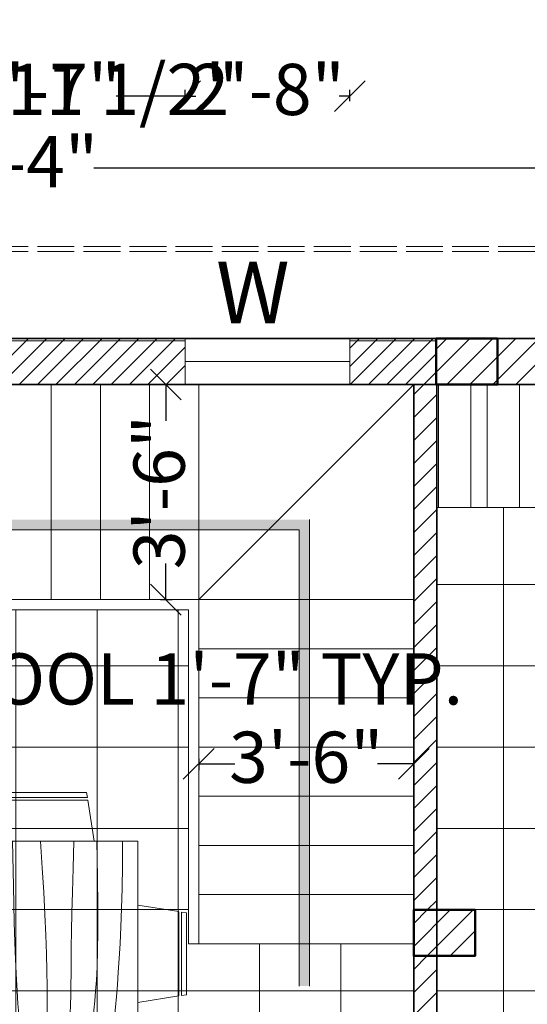
# Model space of a CAD drawing. Units: inches. Extents: x 2036 to 2670, y 319 to 920.
# Tile 11 of 15: x 2350 to 2449, y 728 to 920. Entities that reach past the tile are written whole.
import ezdxf

# ---------------------------------------------------------------- set-up
doc = ezdxf.new("R2010")
doc.units = ezdxf.units.IN
doc.linetypes.add('ACAD_ISO02W100', pattern=[15, 12, -3])
for name, color, linetype, lineweight in [('A-ANNO-DIMS', 2, 'Continuous', 18), ('A-ANNO-SYMB', 7, 'Continuous', 18), ('A-ANNO-SYMB-PATT', 7, 'Continuous', 13), ('A-ANNO-TEXT', 7, 'Continuous', 18), ('A-CASE', 7, 'Continuous', 18), ('A-CASE-PATT', 9, 'Continuous', 13), ('A-COLS', 7, 'Continuous', 50), ('A-FLOR-OVHD', 1, 'ACAD_ISO02W100', 13), ('A-FLOR-PATT', 8, 'Continuous', 9), ('A-FLOR-STRS', 7, 'Continuous', 18), ('A-FURN', 8, 'Continuous', 18), ('A-GLAZ', 4, 'Continuous', 18), ('A-WALL', 7, 'Continuous', 35)]:
    doc.layers.add(name, color=color, linetype=linetype, lineweight=lineweight)
doc.layers.add('A-COLS-PATT', color=240, linetype='Continuous', lineweight=13, true_color=0xed1f24)
doc.layers.add('A-WALL-PATT', color=52, linetype='Continuous', lineweight=13, true_color=0xc8c92d)
doc.styles.get("Standard").update_dxf_attribs({"font": 'arial.ttf'})
doc.dimstyles.new('ISO-25', dxfattribs={"dimtxt": 10, "dimasz": 6, "dimexe": 1.25, "dimexo": 0.625, "dimtad": 0, "dimdec": 1, "dimlunit": 3, "dimtxsty": 'Standard', "dimblk": 'OBLIQUE', "dimcen": 2.5, "dimclrd": 94, "dimclre": 94, "dimclrt": 1, "dimadec": 0, "dimazin": 0, "dimtfac": 1, "dimtdec": 1, "dimtmove": 0, "dimatfit": 3, "dimfxl": 1, "dimfxlon": 1, "dimarcsym": 0})

# ---------------------------------------------------------------- blocks, each defined once
blk = doc.blocks.new('Dining Set - 36 x 72 in.')
for p, q in [((-22, 27.5), (-22.1562, 26.50042)), ((-22, 27.5), (-6, 27.5)), ((-5.8437, 26.49966), (-6, 27.5)), ((6, 27.5), (5.8438, 26.50042)), ((6, 27.5), (22, 27.5)), ((22.1563, 26.49966), (22, 27.5)), ((-22.2343, 26.00059), (-23.4847, 17.99762)), ((-22.2304, 26), (-5.7608, 26)), ((-5.8416, 26.5), (-22.1534, 26.5)), ((-4.5152, 17.99762), (-5.7655, 25.99926)), ((5.7657, 26.00059), (4.5153, 17.99762)), ((5.7696, 26), (22.2392, 26)), ((22.1584, 26.5), (5.8466, 26.5)), ((23.4848, 17.99762), (22.2345, 25.99926)), ((36, 18), (-36, 18)), ((-36, 18), (-36, -18)), ((36, -18), (36, 18)), ((-45.5, 8), (-44.5004, 8.15617)), ((-45.5, 8), (-45.5, -8)), ((-44.5, -8.15843), (-44.5, 8.15338)), ((-44.0006, 8.23428), (-35.9976, 9.48474)), ((-44, 8.23041), (-44, -8.23915)), ((44.0006, 8.23428), (35.9976, 9.48474)), ((44, 8.23041), (44, -8.23915)), ((44.5, -8.15843), (44.5, 8.15338)), ((45.5, 8), (44.5005, 8.15617)), ((45.5, 8), (45.5, -8)), ((-44.4997, -8.15631), (-45.5, -8)), ((-35.9976, -9.48476), (-43.9993, -8.2345)), ((35.9976, -9.48476), (43.9993, -8.2345)), ((44.4997, -8.15631), (45.5, -8)), ((-36, -18), (36, -18)), ((-22.2343, -26.0006), (-23.4847, -17.99762)), ((-4.5152, -17.99762), (-5.7655, -25.99928)), ((5.7657, -26.0006), (4.5153, -17.99762)), ((23.4848, -17.99762), (22.2345, -25.99928)), ((-22.2304, -26), (-5.7608, -26)), ((-22, -27.5), (-22.1562, -26.50044)), ((-5.8416, -26.5), (-22.1534, -26.5)), ((-5.8437, -26.49967), (-6, -27.5)), ((5.7696, -26), (22.2392, -26)), ((6, -27.5), (5.8438, -26.50044)), ((22.1584, -26.5), (5.8466, -26.5)), ((22.1563, -26.49967), (22, -27.5)), ((-22, -27.5), (-6, -27.5)), ((6, -27.5), (22, -27.5))]:
    blk.add_line(p, q)
for points in [[(-36, 15), (-31.1772, 14.97754), (-26.8079, 14.91406), (-22.8538, 14.81543), (-19.276, 14.6875), (-16.0362, 14.53613), (-13.0957, 14.36718), (-10.4159, 14.18652), (-7.9583, 14), (-5.6904, 13.81315), (-3.6035, 13.63021), (-1.6954, 13.45508), (0.0365, 13.29166), (1.5945, 13.14388), (2.9811, 13.01562), (4.1988, 12.9108), (5.25, 12.83333), (6.1393, 12.78613), (6.8802, 12.76823), (7.4883, 12.77767), (7.9792, 12.8125), (8.3685, 12.87077), (8.6719, 12.95052), (8.9049, 13.0498), (9.0833, 13.16666), (9.2205, 13.29899), (9.3216, 13.44401), (9.3895, 13.59879), (9.4271, 13.76041), (9.4373, 13.92594), (9.4232, 14.09245), (9.3875, 14.257), (9.3333, 14.41666), (9.2638, 14.56917), (9.1836, 14.71484), (9.0975, 14.85465), (9.0104, 14.98958), (8.9272, 15.1206), (8.8529, 15.2487), (8.7922, 15.37483), (8.75, 15.5), (8.7305, 15.62467), (8.7344, 15.74739), (8.7617, 15.86621), (8.8125, 15.97916), (8.8867, 16.08431), (8.9844, 16.17968), (9.1055, 16.26334), (9.25, 16.33333), (9.4189, 16.38802), (9.6172, 16.42708), (9.8506, 16.45052), (10.125, 16.45833), (10.4463, 16.45052), (10.8203, 16.42708), (11.2529, 16.38802), (11.75, 16.33333), (12.3184, 16.26318), (12.9694, 16.17838), (13.7151, 16.07991), (14.5677, 15.96875), (15.5395, 15.84586), (16.6426, 15.71224), (17.8893, 15.56884), (19.2917, 15.41666), (20.859, 15.25667), (22.5879, 15.08984), (24.4721, 14.91715), (26.5052, 14.73958), (28.6809, 14.5581), (30.9929, 14.3737), (33.4347, 14.18733), (36, 14)], [(-36, 10), (-28.9766, 10.14274), (-23.1725, 10.20442), (-18.4241, 10.19775), (-14.5677, 10.13541), (-11.4399, 10.03011), (-8.877, 9.89453), (-6.7154, 9.74137), (-4.7917, 9.58333), (-2.9698, 9.43082), (-1.2246, 9.28515), (0.4415, 9.14534), (2.026, 9.01041), (3.5266, 8.87939), (4.9408, 8.7513), (6.266, 8.62516), (7.5, 8.5), (8.6411, 8.37549), (9.6914, 8.2539), (10.6538, 8.13818), (11.5312, 8.03125), (12.3267, 7.93603), (13.043, 7.85547), (13.6831, 7.79248), (14.25, 7.75), (14.7471, 7.7303), (15.1797, 7.73307), (15.5537, 7.75732), (15.875, 7.80208), (16.1494, 7.86637), (16.3828, 7.94922), (16.5811, 8.04964), (16.75, 8.16666), (16.8944, 8.29915), (17.0143, 8.44531), (17.1089, 8.60319), (17.1771, 8.77083), (17.218, 8.94629), (17.2305, 9.1276), (17.2137, 9.31282), (17.1667, 9.5), (17.0895, 9.6875), (16.987, 9.875), (16.8649, 10.0625), (16.7292, 10.25), (16.5856, 10.4375), (16.4401, 10.625), (16.2985, 10.8125), (16.1667, 11), (16.05, 11.18733), (15.9518, 11.3737), (15.8752, 11.5581), (15.8229, 11.73958), (15.798, 11.91715), (15.8034, 12.08984), (15.842, 12.25667), (15.9167, 12.41666), (16.0295, 12.56836), (16.1784, 12.70833), (16.3605, 12.83268), (16.5729, 12.9375), (16.8127, 13.01888), (17.0768, 13.07291), (17.3625, 13.0957), (17.6667, 13.08333), (17.9894, 13.03312), (18.3418, 12.94726), (18.7382, 12.82918), (19.1927, 12.68229), (19.7195, 12.51001), (20.3327, 12.31575), (21.0465, 12.10294), (21.875, 11.875), (22.8357, 11.63354), (23.959, 11.37304), (25.2786, 11.08618), (26.8282, 10.76562), (28.6414, 10.40405), (30.752, 9.99414), (33.1936, 9.52856), (36, 9)], [(-36, 5.5), (-30.7157, 5.3348), (-26.069, 5.20963), (-21.9946, 5.11767), (-18.4271, 5.05208), (-15.3009, 5.00602), (-12.5508, 4.97265), (-10.1112, 4.94515), (-7.9167, 4.91666), (-5.909, 4.88167), (-4.0586, 4.83984), (-2.3429, 4.79215), (-0.7396, 4.73958), (0.7739, 4.6831), (2.22, 4.6237), (3.6213, 4.56233), (5, 4.5), (6.373, 4.43782), (7.7344, 4.3776), (9.0723, 4.32129), (10.375, 4.27083), (11.6309, 4.22819), (12.8281, 4.19531), (13.9551, 4.17415), (15, 4.16666), (15.954, 4.17448), (16.819, 4.19791), (17.6001, 4.23698), (18.3021, 4.29166), (18.9299, 4.36198), (19.4883, 4.44791), (19.9823, 4.54948), (20.4167, 4.66666), (20.7969, 4.79899), (21.1302, 4.94401), (21.4245, 5.09879), (21.6875, 5.26041), (21.9271, 5.42594), (22.1511, 5.59245), (22.3672, 5.757), (22.5834, 5.91666), (22.8065, 6.06868), (23.0404, 6.21093), (23.2879, 6.34147), (23.5521, 6.45833), (23.8358, 6.55957), (24.142, 6.64323), (24.4735, 6.70735), (24.8334, 6.75), (25.2235, 6.76969), (25.642, 6.76692), (26.0858, 6.74267), (26.5521, 6.69791), (27.0379, 6.63362), (27.5404, 6.55078), (28.0565, 6.45036), (28.5834, 6.33333), (29.1242, 6.19987), (29.7071, 6.04687), (30.3661, 5.87044), (31.1354, 5.66666), (32.0493, 5.43164), (33.142, 5.16146), (34.4475, 4.85221), (36, 4.5)], [(-36, -1), (-30.7915, -0.6591), (-26.0195, -0.38216), (-21.6519, -0.16284), (-17.6563, 0.00521), (-14.0005, 0.12833), (-10.6523, 0.21289), (-7.5796, 0.26522), (-4.75, 0.29166), (-2.134, 0.29793), (0.2878, 0.28711), (2.5317, 0.26163), (4.6146, 0.22396), (6.5529, 0.17651), (8.3633, 0.12174), (10.0623, 0.06209), (11.6667, 0), (13.1899, -0.06201), (14.6341, -0.1211), (15.9982, -0.17432), (17.2813, -0.21875), (18.4823, -0.25147), (19.6003, -0.26953), (20.6343, -0.27002), (21.5834, -0.25), (22.4481, -0.20768), (23.2357, -0.14584), (23.9549, -0.06836), (24.6146, 0.02083), (25.2235, 0.11784), (25.7904, 0.21875), (26.3241, 0.31966), (26.8334, 0.41666), (27.3265, 0.50618), (27.8099, 0.58593), (28.2894, 0.65397), (28.7709, 0.70833), (29.2601, 0.74707), (29.763, 0.76823), (30.2855, 0.76985), (30.8334, 0.75), (31.4088, 0.70784), (31.9994, 0.64713), (32.589, 0.57275), (33.1615, 0.48958), (33.7008, 0.4025), (34.1908, 0.3164), (34.6153, 0.23616), (34.9584, 0.16666), (35.2099, 0.11165), (35.3848, 0.07031), (35.504, 0.04069), (35.5886, 0.02083), (35.6594, 0.00879), (35.7377, 0.0026), (35.8442, 0.00032), (36, 0)], [(-36, -6.5), (-27.1843, -6.31267), (-20.084, -6.1263), (-14.469, -5.9419), (-10.1094, -5.76042), (-6.7752, -5.58285), (-4.2363, -5.41016), (-2.2629, -5.24333), (-0.625, -5.08334), (0.8708, -4.93099), (2.2715, -4.78646), (3.5872, -4.64974), (4.8281, -4.52084), (6.0046, -4.39974), (7.127, -4.28646), (8.2053, -4.18099), (9.25, -4.08334), (10.2705, -3.99382), (11.2734, -3.91407), (12.2647, -3.84603), (13.25, -3.79167), (14.2354, -3.75293), (15.2266, -3.73177), (16.2295, -3.73015), (17.25, -3.75), (18.2912, -3.79248), (19.3451, -3.85547), (20.4009, -3.93604), (21.4479, -4.03125), (22.4754, -4.13819), (23.4727, -4.25391), (24.4289, -4.37549), (25.3334, -4.5), (26.1785, -4.62492), (26.9694, -4.74935), (27.7145, -4.87281), (28.4219, -4.99479), (29.1, -5.11483), (29.7572, -5.23242), (30.4016, -5.34709), (31.0417, -5.45834), (31.6837, -5.56437), (32.3262, -5.65821), (32.9658, -5.73153), (33.599, -5.77604), (34.2224, -5.78345), (34.8327, -5.74545), (35.4264, -5.65373), (36, -5.5)], [(-36, -10), (-26.4022, -9.81299), (-18.4675, -9.62891), (-11.9839, -9.45069), (-6.7396, -9.28125), (-2.5226, -9.12354), (0.8789, -8.98047), (3.6769, -8.85498), (6.0833, -8.75), (8.2767, -8.66765), (10.3021, -8.60677), (12.1712, -8.56543), (13.8958, -8.54167), (15.4876, -8.53353), (16.9583, -8.53907), (18.3197, -8.55632), (19.5834, -8.58334), (20.7616, -8.61841), (21.8685, -8.66081), (22.9188, -8.71004), (23.9271, -8.76563), (24.9081, -8.82707), (25.8763, -8.89388), (26.8465, -8.96558), (27.8334, -9.04167), (28.8474, -9.12118), (29.8828, -9.20117), (30.93, -9.27824), (31.9792, -9.34896), (33.0205, -9.40991), (34.0443, -9.45768), (35.0407, -9.48885), (36, -9.5)], [(-36, -14.5), (-30.0881, -14.33513), (-25.0332, -14.21224), (-20.7312, -14.12647), (-17.0781, -14.07292), (-13.97, -14.04671), (-11.3027, -14.04297), (-8.9724, -14.05681), (-6.875, -14.08334), (-4.9224, -14.11833), (-3.0905, -14.16016), (-1.3709, -14.20785), (0.2448, -14.26042), (1.7647, -14.3169), (3.1973, -14.3763), (4.5507, -14.43767), (5.8333, -14.5), (7.0554, -14.5621), (8.235, -14.62175), (9.3922, -14.67652), (10.5469, -14.72396), (11.7192, -14.76164), (12.929, -14.78711), (14.1965, -14.79794), (15.5417, -14.79167), (16.9933, -14.76424), (18.6152, -14.70508), (20.4804, -14.60197), (22.6615, -14.44271), (25.2312, -14.21509), (28.2624, -13.9069), (31.8277, -13.50594), (36, -13)]]:
    blk.add_lwpolyline(points)
blk = doc.blocks.new('_Oblique')
at = {"color": 0, "linetype": 'ByBlock', "lineweight": -2}
blk.add_line((-0.5, -0.5), (0.5, 0.5), dxfattribs=at)
blk = doc.blocks.new('*D10')
at = {"layer": 'A-ANNO-DIMS', "color": 0, "lineweight": -2, "transparency": 16777216}
for p, q in [((2080.74, 889.93), (2080.74, 892.18)), ((2080.74, 890.93), (2328.73, 890.93)), ((2612.74, 890.93), (2364.74, 890.93)), ((2612.74, 889.93), (2612.74, 892.18))]:
    blk.add_line(p, q, dxfattribs=at)
at = {"layer": 'Defpoints', "color": 0, "transparency": 16777216}
for p in [(2612.74, 890.93), (2080.74, 875.68), (2612.74, 875.68)]:
    blk.add_point(p, dxfattribs=at)
at = {"layer": 'A-ANNO-DIMS', "color": 0, "lineweight": -2, "transparency": 16777216, "xscale": 6, "yscale": 6, "zscale": 6, "rotation": 180}
blk.add_blockref('_Oblique', (2080.74, 890.93), dxfattribs=at)
at = {"layer": 'A-ANNO-DIMS', "color": 0, "lineweight": -2, "transparency": 16777216, "xscale": 6, "yscale": 6, "zscale": 6}
blk.add_blockref('_Oblique', (2612.74, 890.93), dxfattribs=at)
at = {"layer": 'A-ANNO-DIMS', "color": 0, "transparency": 16777216, "insert": (2346.74, 890.93), "char_height": 10, "attachment_point": 5}
blk.add_mtext('44\'-4"', dxfattribs=at)
blk = doc.blocks.new('*D16')
at = {"layer": 'A-ANNO-DIMS', "color": 0, "lineweight": -2, "transparency": 16777216}
for p, q in [((2377.81, 848.68), (2380.06, 848.68)), ((2378.81, 848.68), (2378.81, 841.6)), ((2378.81, 806.68), (2378.81, 813.77)), ((2377.81, 806.68), (2380.06, 806.68))]:
    blk.add_line(p, q, dxfattribs=at)
at = {"layer": 'Defpoints', "color": 0, "transparency": 16777216}
for p in [(2375.64, 848.68), (2378.81, 848.68), (2375.64, 806.68)]:
    blk.add_point(p, dxfattribs=at)
at = {"layer": 'A-ANNO-DIMS', "color": 0, "lineweight": -2, "transparency": 16777216, "xscale": 6, "yscale": 6, "zscale": 6}
for p, rotation in [((2378.81, 848.68), 90), ((2378.81, 806.68), 270)]:
    blk.add_blockref('_Oblique', p, dxfattribs=dict(at, rotation=rotation))
at = {"layer": 'A-ANNO-DIMS', "color": 0, "transparency": 16777216, "insert": (2378.81, 827.68), "char_height": 10, "attachment_point": 5, "rotation": 90}
blk.add_mtext('3\'-6"', dxfattribs=at)
blk = doc.blocks.new('*D17')
at = {"layer": 'A-ANNO-DIMS', "color": 0, "lineweight": -2, "transparency": 16777216}
for p, q in [((2385.24, 775.6), (2385.24, 773.35)), ((2427.24, 775.6), (2427.24, 773.35)), ((2385.24, 774.6), (2392.32, 774.6)), ((2427.24, 774.6), (2420.15, 774.6))]:
    blk.add_line(p, q, dxfattribs=at)
at = {"layer": 'Defpoints', "color": 0, "transparency": 16777216}
for p in [(2385.24, 777.88), (2427.24, 777.88), (2427.24, 774.6)]:
    blk.add_point(p, dxfattribs=at)
at = {"layer": 'A-ANNO-DIMS', "color": 0, "lineweight": -2, "transparency": 16777216, "xscale": 6, "yscale": 6, "zscale": 6, "rotation": 180}
blk.add_blockref('_Oblique', (2385.24, 774.6), dxfattribs=at)
at = {"layer": 'A-ANNO-DIMS', "color": 0, "lineweight": -2, "transparency": 16777216, "xscale": 6, "yscale": 6, "zscale": 6}
blk.add_blockref('_Oblique', (2427.24, 774.6), dxfattribs=at)
at = {"layer": 'A-ANNO-DIMS', "color": 0, "transparency": 16777216, "insert": (2406.24, 774.6), "char_height": 10, "attachment_point": 5}
blk.add_mtext('3\'-6"', dxfattribs=at)
blk = doc.blocks.new('COL-9x12')
blk.add_lwpolyline([(9, 0), (0, 0), (0, 12), (9, 12)], close=True)
blk = doc.blocks.new('*D27')
at = {"layer": 'A-ANNO-DIMS', "color": 94, "lineweight": -2, "transparency": 16777216}
for p, q in [((2300.93, 790.9), (2300.93, 788.65)), ((2320.17, 790.9), (2320.17, 788.65)), ((2300.93, 789.9), (2320.17, 789.9)), ((2320.17, 789.9), (2326.17, 789.9))]:
    blk.add_line(p, q, dxfattribs=at)
at = {"layer": 'Defpoints', "color": 0, "transparency": 16777216}
for p in [(2300.93, 792.79), (2320.17, 792.79), (2320.17, 789.9)]:
    blk.add_point(p, dxfattribs=at)
at = {"layer": 'A-ANNO-DIMS', "color": 94, "lineweight": -2, "transparency": 16777216, "xscale": 6, "yscale": 6, "zscale": 6, "rotation": 180}
blk.add_blockref('_Oblique', (2300.93, 789.9), dxfattribs=at)
at = {"layer": 'A-ANNO-DIMS', "color": 94, "lineweight": -2, "transparency": 16777216, "xscale": 6, "yscale": 6, "zscale": 6}
blk.add_blockref('_Oblique', (2320.17, 789.9), dxfattribs=at)
at = {"layer": 'A-ANNO-DIMS', "color": 1, "transparency": 16777216, "insert": (2382.86, 789.9), "char_height": 10, "attachment_point": 5}
blk.add_mtext('STOOL 1\'-7" TYP.', dxfattribs=at)
blk = doc.blocks.new('*D51')
at = {"layer": 'A-ANNO-DIMS', "color": 94, "lineweight": -2, "transparency": 16777216}
for p, q in [((2304.05, 904.03), (2304.05, 906.28)), ((2327.38, 904.03), (2327.38, 906.28)), ((2304.05, 905.03), (2327.38, 905.03)), ((2327.38, 905.03), (2333.38, 905.03))]:
    blk.add_line(p, q, dxfattribs=at)
at = {"layer": 'Defpoints', "color": 0, "transparency": 16777216}
for p in [(2327.38, 905.03), (2304.05, 857.68), (2327.38, 857.68)]:
    blk.add_point(p, dxfattribs=at)
at = {"layer": 'A-ANNO-DIMS', "color": 94, "lineweight": -2, "transparency": 16777216, "xscale": 6, "yscale": 6, "zscale": 6, "rotation": 180}
blk.add_blockref('_Oblique', (2304.05, 905.03), dxfattribs=at)
at = {"layer": 'A-ANNO-DIMS', "color": 94, "lineweight": -2, "transparency": 16777216, "xscale": 6, "yscale": 6, "zscale": 6}
blk.add_blockref('_Oblique', (2327.38, 905.03), dxfattribs=at)
at = {"layer": 'A-ANNO-DIMS', "color": 1, "transparency": 16777216, "insert": (2362.36, 905.03), "char_height": 10, "attachment_point": 5}
blk.add_mtext('1\'-11 1/2"', dxfattribs=at)
blk = doc.blocks.new('*D52')
at = {"layer": 'A-ANNO-DIMS', "color": 94, "lineweight": -2, "transparency": 16777216}
for p, q in [((2327.38, 904.03), (2327.38, 906.28)), ((2382.62, 904.03), (2382.62, 906.28)), ((2327.38, 905.03), (2340.88, 905.03)), ((2382.62, 905.03), (2369.11, 905.03))]:
    blk.add_line(p, q, dxfattribs=at)
at = {"layer": 'Defpoints', "color": 0, "transparency": 16777216}
for p in [(2382.62, 905.03), (2327.38, 857.68), (2382.62, 857.68)]:
    blk.add_point(p, dxfattribs=at)
at = {"layer": 'A-ANNO-DIMS', "color": 94, "lineweight": -2, "transparency": 16777216, "xscale": 6, "yscale": 6, "zscale": 6, "rotation": 180}
blk.add_blockref('_Oblique', (2327.38, 905.03), dxfattribs=at)
at = {"layer": 'A-ANNO-DIMS', "color": 94, "lineweight": -2, "transparency": 16777216, "xscale": 6, "yscale": 6, "zscale": 6}
blk.add_blockref('_Oblique', (2382.62, 905.03), dxfattribs=at)
at = {"layer": 'A-ANNO-DIMS', "color": 1, "transparency": 16777216, "insert": (2355, 905.03), "char_height": 10, "attachment_point": 5}
blk.add_mtext('4\'-7"', dxfattribs=at)
blk = doc.blocks.new('*D53')
at = {"layer": 'A-ANNO-DIMS', "color": 94, "lineweight": -2, "transparency": 16777216}
for p, q in [((2382.62, 904.03), (2382.62, 906.28)), ((2414.79, 904.03), (2414.79, 906.28)), ((2382.62, 905.03), (2384.7, 905.03)), ((2414.79, 905.03), (2412.71, 905.03))]:
    blk.add_line(p, q, dxfattribs=at)
at = {"layer": 'Defpoints', "color": 0, "transparency": 16777216}
for p in [(2414.79, 905.03), (2382.62, 857.68), (2414.79, 857.68)]:
    blk.add_point(p, dxfattribs=at)
at = {"layer": 'A-ANNO-DIMS', "color": 94, "lineweight": -2, "transparency": 16777216, "xscale": 6, "yscale": 6, "zscale": 6, "rotation": 180}
blk.add_blockref('_Oblique', (2382.62, 905.03), dxfattribs=at)
at = {"layer": 'A-ANNO-DIMS', "color": 94, "lineweight": -2, "transparency": 16777216, "xscale": 6, "yscale": 6, "zscale": 6}
blk.add_blockref('_Oblique', (2414.79, 905.03), dxfattribs=at)
at = {"layer": 'A-ANNO-DIMS', "color": 1, "transparency": 16777216, "insert": (2398.7, 905.03), "char_height": 10, "attachment_point": 5}
blk.add_mtext('2\'-8"', dxfattribs=at)

msp = doc.modelspace()

# ---------------------------------------------------------------- hatches: boundary and pattern name
at = {"layer": 'A-ANNO-SYMB-PATT'}
h = msp.add_hatch(color=256, dxfattribs=at)
h.dxf.hatch_style = 1
h.paths.add_polyline_path([(2406.87, 822.33), (2326.91, 822.33), (2326.91, 772.42), (2322.24, 772.42), (2328.91, 764.33), (2328.91, 772.42), (2328.91, 820.33), (2404.87, 820.33), (2404.87, 731.2), (2406.87, 731.2)])
at = {"layer": 'A-CASE-PATT'}
h = msp.add_hatch(dxfattribs=at)
h.set_pattern_fill('ANSI32', color=256, angle=45)
h.paths.add_polyline_path([(2603.74, 848.68), (2431.74, 848.68), (2431.74, 824.68), (2603.74, 824.68)])
at = {"layer": 'A-COLS-PATT'}
h = msp.add_hatch(dxfattribs=at)
h.set_pattern_fill('ANSI31', color=256)
h.paths.add_polyline_path([(2089.74, 875.68), (2080.74, 875.68), (2080.74, 863.68), (2089.74, 863.68)])
h.paths.add_polyline_path([(2089.74, 821.68), (2080.74, 821.68), (2080.74, 809.68), (2089.74, 809.68)])
h.paths.add_polyline_path([(2089.74, 624.2), (2080.74, 624.2), (2080.74, 612.2), (2089.74, 612.2)])
h.paths.add_polyline_path([(2158.74, 506.68), (2149.74, 506.68), (2149.74, 494.68), (2158.74, 494.68)])
h.paths.add_polyline_path([(2158.74, 617.33), (2149.74, 617.33), (2149.74, 605.33), (2158.74, 605.33)])
h.paths.add_polyline_path([(2158.74, 736.18), (2149.74, 736.18), (2149.74, 724.18), (2158.74, 724.18)])
h.paths.add_polyline_path([(2158.74, 852.81), (2149.74, 852.81), (2149.74, 843.81), (2158.74, 843.81)])
h.paths.add_polyline_path([(2161.74, 852.81), (2158.74, 852.81), (2158.74, 843.81), (2161.74, 843.81)])
h.paths.add_polyline_path([(2295.21, 857.66), (2290.74, 857.66), (2290.74, 848.68), (2295.21, 848.68)])
h.paths.add_polyline_path([(2290.74, 857.66), (2283.21, 857.66), (2283.21, 848.66), (2290.74, 848.66)])
h.paths.add_polyline_path([(2443.62, 857.68), (2431.62, 857.68), (2431.62, 848.68), (2443.62, 848.68)])
h.paths.add_polyline_path([(2561.81, 857.68), (2549.81, 857.68), (2549.81, 848.68), (2561.81, 848.68)])
h.paths.add_polyline_path([(2295.24, 737.65), (2290.74, 737.65), (2290.74, 728.68), (2295.24, 728.68)])
h.paths.add_polyline_path([(2309.27, 612.12), (2297.27, 612.12), (2297.27, 603.12), (2309.27, 603.12)])
h.paths.add_polyline_path([(2282.24, 503.68), (2270.24, 503.68), (2270.24, 494.68), (2282.24, 494.68)])
h.paths.add_polyline_path([(2431.74, 746.09), (2427.24, 746.09), (2427.24, 737.09), (2431.74, 737.09)])
h.paths.add_polyline_path([(2439.24, 746.09), (2431.74, 746.09), (2431.74, 737.09), (2439.24, 737.09)])
h.paths.add_polyline_path([(2596.59, 736.59), (2584.59, 736.59), (2584.59, 727.59), (2596.59, 727.59)])
h.paths.add_polyline_path([(2586.39, 623.71), (2574.39, 623.71), (2574.39, 619.18), (2586.39, 619.18)])
h.paths.add_polyline_path([(2586.39, 619.18), (2574.39, 619.18), (2574.39, 614.71), (2586.39, 614.71)])
h.paths.add_polyline_path([(2438.74, 623.68), (2431.24, 623.68), (2431.24, 619.18), (2438.74, 619.18)])
h.paths.add_polyline_path([(2438.74, 619.18), (2431.24, 619.18), (2431.24, 614.68), (2438.74, 614.68)])
h.paths.add_polyline_path([(2431.24, 623.68), (2426.74, 623.68), (2426.74, 614.68), (2431.24, 614.68), (2431.24, 619.18)])
h.paths.add_polyline_path([(2527.24, 503.68), (2515.24, 503.68), (2515.24, 494.68), (2527.24, 494.68)])
h.paths.add_polyline_path([(2590.31, 503.68), (2578.31, 503.68), (2578.31, 494.68), (2590.31, 494.68)])
at = {"layer": 'A-FLOR-PATT'}
h = msp.add_hatch(dxfattribs=at)
h.set_pattern_fill('ANSI31', color=256, scale=5, angle=135)
h.paths.add_polyline_path([(2290.74, 659.68), (2158.74, 659.68), (2158.74, 582.53), (2158.74, 545.51), (2158.74, 503.68), (2426.74, 503.68), (2426.74, 614.68), (2426.74, 623.68), (2426.74, 628.18), (2431.24, 628.18), (2431.24, 623.68), (2438.74, 623.68), (2438.74, 619.18), (2574.39, 619.18), (2574.39, 623.71), (2586.39, 623.71), (2586.39, 619.18), (2603.74, 619.18), (2603.74, 824.68), (2431.74, 824.68), (2431.74, 746.09), (2439.24, 746.09), (2439.24, 737.09), (2431.74, 737.09), (2431.74, 659.68), (2427.24, 659.68), (2427.24, 739.48), (2383.24, 739.48), (2383.24, 804.68), (2339.24, 804.68), (2339.24, 749.08), (2295.24, 749.08), (2295.24, 737.65), (2295.27, 737.65), (2295.27, 728.65), (2295.21, 728.65, -0.586418), (2272.74, 728.68), (2272.74, 824.68), (2270.11, 824.68), (2270.11, 829.18), (2290.74, 829.18), (2290.74, 848.66), (2283.21, 848.66), (2283.21, 857.66), (2289.74, 857.66), (2289.74, 874.68), (2158.74, 874.68), (2158.74, 852.81), (2161.74, 852.81), (2161.74, 843.81), (2158.74, 843.81), (2158.74, 829.18), (2224.74, 829.18), (2224.74, 800.68), (2182.74, 800.68), (2182.74, 733.41), (2158.74, 733.41), (2158.74, 728.68), (2235.24, 728.68), (2235.24, 714.81), (2230.74, 714.81), (2230.74, 724.18), (2158.74, 724.18), (2158.74, 664.18), (2230.74, 664.18), (2230.74, 678.81), (2235.24, 678.81), (2235.24, 664.18), (2290.74, 664.18)])
h.paths.add_polyline_path([(2309.27, 612.12), (2309.27, 603.12), (2297.27, 603.12), (2297.27, 612.12)], flags=16)
h.paths.add_polyline_path([(2280.12, 639.11), (2280.26, 638.18, -0.414214), (2279.26, 637.18), (2278.76, 637.18), (2279.26, 633.18), (2277.76, 633.18), (2277.26, 637.18), (2269.76, 637.18), (2262.26, 637.18), (2261.76, 633.18), (2260.26, 633.18), (2260.76, 637.18), (2260.26, 637.18, -0.414214), (2259.26, 638.18), (2259.41, 639.11, -0.541164), (2257.76, 641.18), (2260.76, 652.18), (2261.45, 652.18), (2261.53, 652.68), (2262.76, 652.68), (2262.25, 655.24, 0.001913), (2261.76, 655.18), (2259.76, 658.18, -0.15), (2279.76, 658.18), (2277.76, 655.18, 0.001913), (2277.27, 655.24), (2276.76, 652.68), (2278, 652.68), (2278.07, 652.18), (2278.76, 652.18), (2281.76, 641.18, -0.541163)], flags=16)
h.paths.add_polyline_path([(2245.98, 639.11), (2246.13, 638.18, -0.414214), (2245.13, 637.18), (2244.63, 637.18), (2245.13, 633.18), (2243.63, 633.18), (2243.13, 637.18), (2235.63, 637.18), (2228.13, 637.18), (2227.63, 633.18), (2226.13, 633.18), (2226.63, 637.18), (2226.13, 637.18, -0.414214), (2225.13, 638.18), (2225.27, 639.11, -0.541164), (2223.63, 641.18), (2226.63, 652.18), (2227.32, 652.18), (2227.39, 652.68), (2228.63, 652.68), (2228.12, 655.24, 0.001913), (2227.63, 655.18), (2225.63, 658.18, -0.15), (2245.63, 658.18), (2243.63, 655.18, 0.001913), (2243.14, 655.24), (2242.63, 652.68), (2243.86, 652.68), (2243.94, 652.18), (2244.63, 652.18), (2247.63, 641.18, -0.541163)], flags=16)
h.paths.add_polyline_path([(2351.59, 515.15, -0.151948), (2279.59, 515.15), (2279.59, 537.68), (2273.59, 537.68), (2273.59, 511.68, 0.190476), (2357.59, 511.68), (2357.59, 537.68), (2351.59, 537.68)])
h.paths.add_polyline_path([(2327.59, 536.13), (2327.59, 517.07), (2303.59, 517.07), (2303.59, 536.13)], flags=16)
h.paths.add_polyline_path([(2213.4, 639.11), (2213.55, 638.18, -0.414214), (2212.55, 637.18), (2212.05, 637.18), (2212.55, 633.18), (2211.05, 633.18), (2210.55, 637.18), (2203.05, 637.18), (2195.55, 637.18), (2195.05, 633.18), (2193.55, 633.18), (2194.05, 637.18), (2193.55, 637.18, -0.414214), (2192.55, 638.18), (2192.69, 639.11, -0.541164), (2191.05, 641.18), (2194.05, 652.18), (2194.73, 652.18), (2194.81, 652.68), (2196.05, 652.68), (2195.53, 655.24, 0.001913), (2195.05, 655.18), (2193.05, 658.18, -0.15), (2213.05, 658.18), (2211.05, 655.18, 0.001913), (2210.56, 655.24), (2210.05, 652.68), (2211.28, 652.68), (2211.36, 652.18), (2212.05, 652.18), (2215.05, 641.18, -0.541163)], flags=16)
h.paths.add_polyline_path([(2368.58, 538.02), (2370.52, 538.02), (2371.17, 532.84), (2380.89, 532.84), (2390.6, 532.84), (2391.25, 538.02), (2393.2, 538.02), (2392.55, 532.84), (2380.89, 532.84), (2368.58, 532.84, 0.414214), (2367.28, 531.54), (2367.47, 530.34, -0.483352), (2369.23, 527.65), (2371.82, 513.4), (2370.12, 513.4), (2370.22, 512.75), (2391.56, 512.75), (2391.66, 513.4), (2389.96, 513.4), (2392.55, 527.65, -1.387427), (2396.43, 527.65), (2392.55, 513.4), (2391.66, 513.4), (2391.56, 512.75), (2389.31, 512.75), (2390, 509.37, 0.003796), (2391.25, 509.51), (2393.84, 505.63, -0.15), (2367.93, 505.63), (2370.52, 509.51, 0.003901), (2371.81, 509.36), (2372.47, 512.75), (2370.22, 512.75), (2370.12, 513.4), (2369.23, 513.4), (2365.34, 527.65, -0.541163), (2367.47, 530.34), (2367.28, 531.54, -0.414214), (2368.58, 532.84), (2369.23, 532.84)])
h.paths.add_polyline_path([(2266.74, 538.02), (2266.09, 532.84), (2254.43, 532.84), (2242.12, 532.84, 0.414214), (2240.83, 531.54), (2241.01, 530.34, -0.483352), (2242.77, 527.65), (2245.36, 513.4), (2243.66, 513.4), (2243.76, 512.75), (2265.1, 512.75), (2265.2, 513.4), (2263.5, 513.4), (2266.09, 527.65, -1.387427), (2269.98, 527.65), (2266.09, 513.4), (2265.2, 513.4), (2265.1, 512.75), (2262.85, 512.75), (2263.54, 509.37, 0.003796), (2264.79, 509.51), (2267.39, 505.63, -0.15), (2241.47, 505.63), (2244.07, 509.51, 0.003901), (2245.36, 509.36), (2246.01, 512.75), (2243.76, 512.75), (2243.66, 513.4), (2242.77, 513.4), (2238.88, 527.65, -0.541163), (2241.01, 530.34), (2240.83, 531.54, -0.414214), (2242.12, 532.84), (2242.77, 532.84), (2242.12, 538.02), (2244.07, 538.02), (2244.71, 532.84), (2254.43, 532.84), (2264.15, 532.84), (2264.79, 538.02)])
h.paths.add_polyline_path([(2185.24, 620.36), (2185.24, 618.86), (2181.24, 618.36), (2181.24, 610.86), (2181.24, 603.36), (2185.24, 602.86), (2185.24, 601.36), (2181.24, 601.86), (2181.24, 601.36, -0.414214), (2180.24, 600.36), (2179.31, 600.5, -0.541164), (2177.24, 598.86), (2166.24, 601.86), (2166.24, 602.54), (2165.74, 602.62), (2165.74, 603.86), (2163.18, 603.34, 0.001913), (2163.24, 602.86), (2160.24, 600.86, -0.15), (2160.24, 620.86), (2163.24, 618.86, 0.001913), (2163.18, 618.37), (2165.74, 617.86), (2165.74, 619.09), (2166.24, 619.17), (2166.24, 619.86), (2177.24, 622.86, -0.541163), (2179.31, 621.21), (2180.24, 621.36, -0.414214), (2181.24, 620.36), (2181.24, 619.86)])
h.paths.add_polyline_path([(2470.92, 676.01), (2470.92, 806.13), (2568.52, 806.13), (2568.52, 676.01)], flags=16)
h.paths.add_polyline_path([(2177.74, 677.49), (2161.9, 677.49), (2161.9, 705.85), (2177.74, 705.85)], flags=16)
h.paths.add_polyline_path([(2176.74, 678.49), (2162.9, 678.49), (2162.9, 704.85), (2176.74, 704.85)], flags=0)
h.paths.add_polyline_path([(2175.01, 686.48), (2172.93, 686.48), (2172.93, 690.63), (2170.86, 690.63), (2170.86, 686.48), (2164.63, 686.48), (2164.63, 688.56), (2166.71, 688.56), (2168.78, 688.56), (2168.78, 690.63), (2164.63, 690.63), (2164.63, 696.85), (2166.71, 696.85), (2166.71, 692.71), (2168.78, 692.71), (2168.78, 696.85), (2175.01, 696.85), (2175.01, 694.78), (2170.86, 694.78), (2170.86, 692.71), (2175.01, 692.71)], flags=0)
h.paths.add_polyline_path([(2543.79, 782.71), (2483.94, 782.71), (2483.94, 804.18), (2517.77, 804.18), (2517.77, 782.71), (2521.67, 782.71), (2521.67, 804.18), (2555.5, 804.18), (2555.5, 779.45), (2547.05, 779.45), (2568.52, 757.98), (2543.79, 757.98)], flags=0)
h.paths.add_polyline_path([(2584.59, 727.59), (2584.59, 736.59), (2596.59, 736.59), (2596.59, 727.59)], flags=16)
h.paths.add_polyline_path([(2520.45, 647.03), (2553.79, 647.03), (2553.79, 658.23), (2520.45, 658.23)], flags=24)
h.paths.add_polyline_path([(2299.53, 573.74), (2331.71, 573.74), (2331.71, 584.94), (2299.53, 584.94)], flags=24)
h.paths.add_polyline_path([(2191.59, 685.19), (2212.12, 685.19), (2212.12, 696.38), (2191.59, 696.38)], flags=24)
h.paths.add_polyline_path([(2353.9, 649.86), (2379.08, 649.86), (2379.08, 661.06), (2353.9, 661.06)], flags=24)
h.paths.add_polyline_path([(2214.61, 763.31), (2237.46, 763.31), (2237.46, 779.56), (2214.61, 779.56)], flags=24)
h.paths.add_polyline_path([(2225.09, 819.31), (2269.29, 819.31), (2269.29, 844.04), (2225.09, 844.04)], flags=24)
h.paths.add_polyline_path([(2204.06, 845.04), (2226.92, 845.04), (2226.92, 856.24), (2204.06, 856.24)], flags=24)
h = msp.add_hatch(dxfattribs=at)
h.set_pattern_fill('ANSI31', color=256, scale=5, angle=45)
h.paths.add_polyline_path([(2290.74, 659.68), (2158.74, 659.68), (2158.74, 582.53), (2158.74, 545.51), (2158.74, 503.68), (2426.74, 503.68), (2426.74, 614.68), (2426.74, 623.68), (2426.74, 628.18), (2431.24, 628.18), (2431.24, 623.68), (2438.74, 623.68), (2438.74, 619.18), (2574.39, 619.18), (2574.39, 623.71), (2586.39, 623.71), (2586.39, 619.18), (2603.74, 619.18), (2603.74, 824.68), (2431.74, 824.68), (2431.74, 746.09), (2439.24, 746.09), (2439.24, 737.09), (2431.74, 737.09), (2431.74, 659.68), (2427.24, 659.68), (2427.24, 739.48), (2383.24, 739.48), (2383.24, 804.68), (2339.24, 804.68), (2339.24, 749.08), (2295.24, 749.08), (2295.24, 737.65), (2295.27, 737.65), (2295.27, 728.65), (2295.21, 728.65, -0.586418), (2272.74, 728.68), (2272.74, 824.68), (2270.11, 824.68), (2270.11, 829.18), (2290.74, 829.18), (2290.74, 848.66), (2283.21, 848.66), (2283.21, 857.66), (2289.74, 857.66), (2289.74, 874.68), (2158.74, 874.68), (2158.74, 852.81), (2161.74, 852.81), (2161.74, 843.81), (2158.74, 843.81), (2158.74, 829.18), (2224.74, 829.18), (2224.74, 800.68), (2182.74, 800.68), (2182.74, 733.41), (2158.74, 733.41), (2158.74, 728.68), (2235.24, 728.68), (2235.24, 714.81), (2230.74, 714.81), (2230.74, 724.18), (2158.74, 724.18), (2158.74, 664.18), (2230.74, 664.18), (2230.74, 678.81), (2235.24, 678.81), (2235.24, 664.18), (2290.74, 664.18)])
h.paths.add_polyline_path([(2309.27, 612.12), (2309.27, 603.12), (2297.27, 603.12), (2297.27, 612.12)], flags=16)
h.paths.add_polyline_path([(2280.12, 639.11), (2280.26, 638.18, -0.414214), (2279.26, 637.18), (2278.76, 637.18), (2279.26, 633.18), (2277.76, 633.18), (2277.26, 637.18), (2269.76, 637.18), (2262.26, 637.18), (2261.76, 633.18), (2260.26, 633.18), (2260.76, 637.18), (2260.26, 637.18, -0.414214), (2259.26, 638.18), (2259.41, 639.11, -0.541164), (2257.76, 641.18), (2260.76, 652.18), (2261.45, 652.18), (2261.53, 652.68), (2262.76, 652.68), (2262.25, 655.24, 0.001913), (2261.76, 655.18), (2259.76, 658.18, -0.15), (2279.76, 658.18), (2277.76, 655.18, 0.001913), (2277.27, 655.24), (2276.76, 652.68), (2278, 652.68), (2278.07, 652.18), (2278.76, 652.18), (2281.76, 641.18, -0.541163)], flags=16)
h.paths.add_polyline_path([(2245.98, 639.11), (2246.13, 638.18, -0.414214), (2245.13, 637.18), (2244.63, 637.18), (2245.13, 633.18), (2243.63, 633.18), (2243.13, 637.18), (2235.63, 637.18), (2228.13, 637.18), (2227.63, 633.18), (2226.13, 633.18), (2226.63, 637.18), (2226.13, 637.18, -0.414214), (2225.13, 638.18), (2225.27, 639.11, -0.541164), (2223.63, 641.18), (2226.63, 652.18), (2227.32, 652.18), (2227.39, 652.68), (2228.63, 652.68), (2228.12, 655.24, 0.001913), (2227.63, 655.18), (2225.63, 658.18, -0.15), (2245.63, 658.18), (2243.63, 655.18, 0.001913), (2243.14, 655.24), (2242.63, 652.68), (2243.86, 652.68), (2243.94, 652.18), (2244.63, 652.18), (2247.63, 641.18, -0.541163)], flags=16)
h.paths.add_polyline_path([(2351.59, 537.68), (2351.59, 515.15, -0.151948), (2279.59, 515.15), (2279.59, 537.68), (2273.59, 537.68), (2273.59, 511.68, 0.190476), (2357.59, 511.68), (2357.59, 537.68)])
h.paths.add_polyline_path([(2368.58, 538.02), (2370.52, 538.02), (2371.17, 532.84), (2380.89, 532.84), (2390.6, 532.84), (2391.25, 538.02), (2393.2, 538.02), (2392.55, 532.84), (2380.89, 532.84), (2368.58, 532.84, 0.414214), (2367.28, 531.54), (2367.47, 530.34, -0.483352), (2369.23, 527.65), (2371.82, 513.4), (2370.12, 513.4), (2370.22, 512.75), (2391.56, 512.75), (2391.66, 513.4), (2389.96, 513.4), (2392.55, 527.65, -1.387427), (2396.43, 527.65), (2392.55, 513.4), (2391.66, 513.4), (2391.56, 512.75), (2389.31, 512.75), (2390, 509.37, 0.003796), (2391.25, 509.51), (2393.84, 505.63, -0.15), (2367.93, 505.63), (2370.52, 509.51, 0.003901), (2371.81, 509.36), (2372.47, 512.75), (2370.22, 512.75), (2370.12, 513.4), (2369.23, 513.4), (2365.34, 527.65, -0.541163), (2367.47, 530.34), (2367.28, 531.54, -0.414214), (2368.58, 532.84), (2369.23, 532.84)])
h.paths.add_polyline_path([(2327.59, 536.13), (2327.59, 517.07), (2303.59, 517.07), (2303.59, 536.13)], flags=16)
h.paths.add_polyline_path([(2470.92, 676.01), (2470.92, 806.13), (2568.52, 806.13), (2568.52, 676.01)], flags=16)
h.paths.add_polyline_path([(2266.74, 538.02), (2266.09, 532.84), (2254.43, 532.84), (2242.12, 532.84, 0.414214), (2240.83, 531.54), (2241.01, 530.34, -0.483352), (2242.77, 527.65), (2245.36, 513.4), (2243.66, 513.4), (2243.76, 512.75), (2265.1, 512.75), (2265.2, 513.4), (2263.5, 513.4), (2266.09, 527.65, -1.387427), (2269.98, 527.65), (2266.09, 513.4), (2265.2, 513.4), (2265.1, 512.75), (2262.85, 512.75), (2263.54, 509.37, 0.003796), (2264.79, 509.51), (2267.39, 505.63, -0.15), (2241.47, 505.63), (2244.07, 509.51, 0.003901), (2245.36, 509.36), (2246.01, 512.75), (2243.76, 512.75), (2243.66, 513.4), (2242.77, 513.4), (2238.88, 527.65, -0.541163), (2241.01, 530.34), (2240.83, 531.54, -0.414214), (2242.12, 532.84), (2242.77, 532.84), (2242.12, 538.02), (2244.07, 538.02), (2244.71, 532.84), (2254.43, 532.84), (2264.15, 532.84), (2264.79, 538.02)])
h.paths.add_polyline_path([(2213.4, 639.11), (2213.55, 638.18, -0.414214), (2212.55, 637.18), (2212.05, 637.18), (2212.55, 633.18), (2211.05, 633.18), (2210.55, 637.18), (2203.05, 637.18), (2195.55, 637.18), (2195.05, 633.18), (2193.55, 633.18), (2194.05, 637.18), (2193.55, 637.18, -0.414214), (2192.55, 638.18), (2192.69, 639.11, -0.541164), (2191.05, 641.18), (2194.05, 652.18), (2194.73, 652.18), (2194.81, 652.68), (2196.05, 652.68), (2195.53, 655.24, 0.001913), (2195.05, 655.18), (2193.05, 658.18, -0.15), (2213.05, 658.18), (2211.05, 655.18, 0.001913), (2210.56, 655.24), (2210.05, 652.68), (2211.28, 652.68), (2211.36, 652.18), (2212.05, 652.18), (2215.05, 641.18, -0.541163)], flags=16)
h.paths.add_polyline_path([(2185.24, 620.36), (2185.24, 618.86), (2181.24, 618.36), (2181.24, 610.86), (2181.24, 603.36), (2185.24, 602.86), (2185.24, 601.36), (2181.24, 601.86), (2181.24, 601.36, -0.414214), (2180.24, 600.36), (2179.31, 600.5, -0.541164), (2177.24, 598.86), (2166.24, 601.86), (2166.24, 602.54), (2165.74, 602.62), (2165.74, 603.86), (2163.18, 603.34, 0.001913), (2163.24, 602.86), (2160.24, 600.86, -0.15), (2160.24, 620.86), (2163.24, 618.86, 0.001913), (2163.18, 618.37), (2165.74, 617.86), (2165.74, 619.09), (2166.24, 619.17), (2166.24, 619.86), (2177.24, 622.86, -0.541163), (2179.31, 621.21), (2180.24, 621.36, -0.414214), (2181.24, 620.36), (2181.24, 619.86)])
h.paths.add_polyline_path([(2177.74, 677.49), (2161.9, 677.49), (2161.9, 705.85), (2177.74, 705.85)], flags=16)
h.paths.add_polyline_path([(2176.74, 678.49), (2162.9, 678.49), (2162.9, 704.85), (2176.74, 704.85)], flags=0)
h.paths.add_polyline_path([(2175.01, 686.48), (2172.93, 686.48), (2172.93, 690.63), (2170.86, 690.63), (2170.86, 686.48), (2164.63, 686.48), (2164.63, 688.56), (2166.71, 688.56), (2168.78, 688.56), (2168.78, 690.63), (2164.63, 690.63), (2164.63, 696.85), (2166.71, 696.85), (2166.71, 692.71), (2168.78, 692.71), (2168.78, 696.85), (2175.01, 696.85), (2175.01, 694.78), (2170.86, 694.78), (2170.86, 692.71), (2175.01, 692.71)], flags=0)
h.paths.add_polyline_path([(2543.79, 782.71), (2483.94, 782.71), (2483.94, 804.18), (2517.77, 804.18), (2517.77, 782.71), (2521.67, 782.71), (2521.67, 804.18), (2555.5, 804.18), (2555.5, 779.45), (2547.05, 779.45), (2568.52, 757.98), (2543.79, 757.98)], flags=0)
h.paths.add_polyline_path([(2584.59, 727.59), (2584.59, 736.59), (2596.59, 736.59), (2596.59, 727.59)], flags=16)
h.paths.add_polyline_path([(2520.45, 647.03), (2553.79, 647.03), (2553.79, 658.23), (2520.45, 658.23)], flags=24)
h.paths.add_polyline_path([(2299.53, 573.74), (2331.71, 573.74), (2331.71, 584.94), (2299.53, 584.94)], flags=24)
h.paths.add_polyline_path([(2191.59, 685.19), (2212.12, 685.19), (2212.12, 696.38), (2191.59, 696.38)], flags=24)
h.paths.add_polyline_path([(2353.9, 649.86), (2379.08, 649.86), (2379.08, 661.06), (2353.9, 661.06)], flags=24)
h.paths.add_polyline_path([(2214.61, 763.31), (2237.46, 763.31), (2237.46, 779.56), (2214.61, 779.56)], flags=24)
h.paths.add_polyline_path([(2225.09, 819.31), (2269.29, 819.31), (2269.29, 844.04), (2225.09, 844.04)], flags=24)
h.paths.add_polyline_path([(2204.06, 845.04), (2226.92, 845.04), (2226.92, 856.24), (2204.06, 856.24)], flags=24)
at = {"layer": 'A-WALL-PATT'}
h = msp.add_hatch(dxfattribs=at)
h.set_pattern_fill('ANSI31', color=256)
h.paths.add_polyline_path([(2089.74, 863.68), (2080.74, 863.68), (2080.74, 821.68), (2089.74, 821.68)])
h.paths.add_polyline_path([(2089.74, 809.68), (2080.74, 809.68), (2080.74, 624.2), (2089.74, 624.2), (2089.74, 707.68), (2089.74, 767.68)])
h.paths.add_polyline_path([(2149.74, 818.68), (2089.74, 818.68), (2089.74, 809.68), (2149.74, 809.68)])
h.paths.add_polyline_path([(2158.74, 875.68), (2089.74, 875.68), (2089.74, 866.68), (2149.74, 866.68), (2149.74, 852.81), (2158.74, 852.81)])
h.paths.add_polyline_path([(2158.74, 843.81), (2149.74, 843.81), (2149.74, 736.18), (2158.74, 736.18), (2158.74, 824.68)])
h.paths.add_polyline_path([(2181.31, 829.18), (2158.74, 829.18), (2158.74, 824.68), (2181.31, 824.68)])
h.paths.add_polyline_path([(2224.74, 829.18), (2212.72, 829.18), (2212.72, 824.68), (2224.74, 824.68)])
h.paths.add_polyline_path([(2177.02, 503.68), (2158.74, 503.68), (2158.74, 494.68), (2177.02, 494.68)])
h.paths.add_polyline_path([(2158.74, 664.18), (2158.74, 680.02), (2149.74, 680.02), (2149.74, 617.33), (2158.74, 617.33)])
h.paths.add_polyline_path([(2158.74, 724.18), (2149.74, 724.18), (2149.74, 704.02), (2158.74, 704.02)])
h.paths.add_polyline_path([(2235.24, 728.68), (2158.74, 728.68), (2158.74, 724.18), (2230.74, 724.18), (2230.74, 714.81), (2235.24, 714.81)])
h.paths.add_polyline_path([(2290.74, 664.18), (2235.24, 664.18), (2235.24, 678.81), (2230.74, 678.81), (2230.74, 664.18), (2158.74, 664.18), (2158.74, 659.68), (2290.74, 659.68)])
h.paths.add_polyline_path([(2270.24, 503.68), (2227.17, 503.68), (2227.17, 494.68), (2270.24, 494.68)])
h.paths.add_polyline_path([(2515.24, 503.68), (2380.89, 503.68), (2380.89, 494.68), (2515.24, 494.68)])
h.paths.add_polyline_path([(2292.21, 503.68), (2282.24, 503.68), (2282.24, 494.68), (2292.21, 494.68)])
h.paths.add_polyline_path([(2578.31, 503.68), (2527.24, 503.68), (2527.24, 494.68), (2578.31, 494.68)])
h.paths.add_polyline_path([(2603.74, 503.68), (2590.31, 503.68), (2590.31, 494.68), (2603.74, 494.68)])
h.paths.add_polyline_path([(2612.74, 503.68), (2603.74, 503.68), (2603.74, 494.68), (2612.74, 494.68)])
h.paths.add_polyline_path([(2549.81, 857.68), (2443.62, 857.68), (2443.62, 848.68), (2549.81, 848.68)])
h.paths.add_polyline_path([(2295.24, 848.66), (2290.74, 848.66), (2290.74, 829.18), (2270.11, 829.18), (2270.11, 824.68), (2290.74, 824.68), (2290.74, 737.65), (2295.24, 737.65)])
h.paths.add_polyline_path([(2431.74, 737.09), (2427.24, 737.09), (2427.24, 659.68), (2431.74, 659.68)])
h.paths.add_polyline_path([(2431.74, 848.68), (2427.24, 848.68), (2427.24, 746.09), (2431.74, 746.09)])
h.paths.add_polyline_path([(2574.39, 619.18), (2495.46, 619.18), (2495.46, 614.68), (2574.39, 614.68)])
h.paths.add_polyline_path([(2461.84, 619.18), (2438.74, 619.18), (2438.74, 614.68), (2461.84, 614.68)])
h.paths.add_polyline_path([(2603.74, 619.18), (2586.39, 619.18), (2586.39, 614.68), (2603.74, 614.68)], flags=17)
h = msp.add_hatch(dxfattribs=at)
h.set_pattern_fill('ANSI31', color=256, scale=3, angle=135)
h.paths.add_polyline_path([(2382.62, 857.68), (2327.38, 857.68), (2327.38, 848.68), (2382.62, 848.68)])
h.paths.add_polyline_path([(2431.62, 857.68), (2414.79, 857.68), (2414.79, 848.68), (2427.24, 848.68), (2431.62, 848.68)])
h = msp.add_hatch(dxfattribs=at)
h.set_pattern_fill('ANSI31', color=256, scale=0.8)
h.paths.add_polyline_path([(2431.62, 857.68), (2414.79, 857.68), (2414.79, 848.68), (2427.24, 848.68), (2431.62, 848.68)])
h.paths.add_polyline_path([(2382.62, 857.68), (2327.38, 857.68), (2327.38, 848.68), (2382.62, 848.68)])
h = msp.add_hatch(dxfattribs=at)
h.set_pattern_fill('ANSI31', color=256, scale=3, angle=135)
h.paths.add_polyline_path([(2431.62, 857.68), (2414.79, 857.68), (2414.79, 848.68), (2427.24, 848.68), (2431.62, 848.68)])

# ---------------------------------------------------------------- linework, layer by layer
at = {"layer": 'A-ANNO-SYMB'}
for p, q in [((2406.87, 731.2), (2406.87, 822.33)), ((2404.87, 820.33), (2328.91, 820.33)), ((2404.87, 731.2), (2404.87, 820.33))]:
    msp.add_line(p, q, dxfattribs=at)
at = {"layer": 'A-CASE'}
msp.add_line((2603.74, 824.68), (2431.74, 824.68), dxfattribs=at)
at = {"layer": 'A-COLS'}
msp.add_lwpolyline([(2443.62, 857.68), (2443.62, 848.68), (2431.62, 848.68), (2431.62, 857.68)], close=True, dxfattribs=at)
at = {"layer": 'A-FLOR-OVHD', "ltscale": 0.6}
for p, q in [((2290.74, 875.68), (2612.74, 875.68)), ((2290.74, 874.68), (2612.74, 874.68))]:
    msp.add_line(p, q, dxfattribs=at)
at = {"layer": 'A-FLOR-STRS'}
for p, q in [((2356.44, 806.68), (2356.44, 848.68)), ((2366.04, 806.68), (2366.04, 848.68)), ((2375.64, 806.68), (2375.64, 848.68)), ((2385.24, 806.68), (2385.24, 848.68)), ((2385.24, 806.68), (2427.24, 848.68)), ((2427.24, 806.68), (2385.24, 806.68)), ((2427.24, 797.08), (2385.24, 797.08)), ((2427.24, 787.48), (2385.24, 787.48)), ((2427.24, 777.88), (2385.24, 777.88)), ((2427.24, 768.28), (2385.24, 768.28)), ((2427.24, 758.68), (2385.24, 758.68)), ((2427.24, 749.08), (2385.24, 749.08)), ((2427.24, 739.48), (2383.24, 739.48))]:
    msp.add_line(p, q, dxfattribs=at)
for points in [[(2385.24, 739.48), (2385.24, 806.68), (2337.24, 806.68), (2337.24, 749.08)], [(2383.24, 739.48), (2383.24, 804.68), (2339.24, 804.68), (2339.24, 749.08)]]:
    msp.add_lwpolyline(points, dxfattribs=at)
at = {"layer": 'A-GLAZ'}
for p, q in [((2382.62, 857.68), (2382.62, 848.68)), ((2414.79, 857.68), (2414.79, 848.68)), ((2382.62, 853.18), (2414.79, 853.18))]:
    msp.add_line(p, q, dxfattribs=at)
at = {"layer": 'A-WALL'}
for p, q in [((2612.74, 857.68), (2290.74, 857.68)), ((2427.24, 848.68), (2295.24, 848.68)), ((2427.24, 659.68), (2427.24, 848.68)), ((2431.74, 848.68), (2427.24, 848.68)), ((2603.74, 848.68), (2431.74, 848.68)), ((2431.74, 659.68), (2431.74, 848.68))]:
    msp.add_line(p, q, dxfattribs=at)

# ---------------------------------------------------------------- block references
at = {"layer": 'A-COLS', "rotation": 89.9999999999986}
msp.add_blockref('COL-9x12', (2439.24, 737.09), dxfattribs=at)
at = {"layer": 'A-FURN', "rotation": 270}
msp.add_blockref('Dining Set - 36 x 72 in.', (2355.36, 723.51), dxfattribs=at)

# ---------------------------------------------------------------- texts
at = {"layer": 'A-ANNO-TEXT', "insert": (2388.63, 872.67), "char_height": 12, "attachment_point": 1}
msp.add_mtext_dynamic_manual_height_columns('W', width=27.6972, gutter_width=12.5, heights=[0], dxfattribs=at)

# ---------------------------------------------------------------- dimensions: what is measured, and where the dimension line sits
at = {"layer": 'A-ANNO-DIMS'}
for base, p1, p2, override, picture, middle in [((2327.38, 905.03), (2304.05, 857.68), (2327.38, 857.68), {"dimdec": 1, "dimlfac": 1, "dimrnd": 0, "dimzin": 1, "dimdsep": 46, "dimlunit": 4, "dimfrac": 2}, '*D51', (2362.36, 905.03)), ((2382.62, 905.03), (2327.38, 857.68), (2382.62, 857.68), {"dimdec": 1, "dimlfac": 1, "dimrnd": 0, "dimzin": 1, "dimdsep": 46, "dimlunit": 4, "dimfrac": 2}, '*D52', (2355, 905.03)), ((2414.79, 905.03), (2382.62, 857.68), (2414.79, 857.68), {"dimdec": 1, "dimlfac": 1, "dimrnd": 0, "dimzin": 1, "dimdsep": 46, "dimlunit": 4, "dimfrac": 2}, '*D53', (2398.7, 905.03)), ((2612.74, 890.93), (2080.74, 875.68), (2612.74, 875.68), {"dimclrd": 0, "dimclre": 0, "dimclrt": 0}, '*D10', (2346.74, 890.93)), ((2427.24, 774.6), (2385.24, 777.88), (2427.24, 777.88), {"dimclrd": 0, "dimclre": 0, "dimclrt": 0}, '*D17', (2406.24, 774.6))]:
    dim = msp.add_linear_dim(base=base, p1=p1, p2=p2, dimstyle='ISO-25', override=override, dxfattribs=at)
    dim.commit()
    dim.dimension.update_dxf_attribs({"geometry": picture, "text_midpoint": middle})
dim = msp.add_linear_dim(base=(2378.81, 848.68), p1=(2375.64, 806.68), p2=(2375.64, 848.68), angle=90, dimstyle='ISO-25', override={"dimclrd": 0, "dimclre": 0, "dimclrt": 0}, dxfattribs=at)
dim.commit()
dim.dimension.update_dxf_attribs({"geometry": '*D16', "text_midpoint": (2378.81, 827.68)})
dim = msp.add_linear_dim(base=(2320.17, 789.9), p1=(2300.93, 792.79), p2=(2320.17, 792.79), text='STOOL <> TYP.', dimstyle='ISO-25', override={"dimdec": 1, "dimlfac": 1, "dimrnd": 0, "dimzin": 1, "dimdsep": 46, "dimlunit": 4, "dimfrac": 2}, dxfattribs=at)
dim.commit()
dim.dimension.update_dxf_attribs({"geometry": '*D27', "text_midpoint": (2382.86, 789.9)})

doc.saveas('drawing.dxf')
